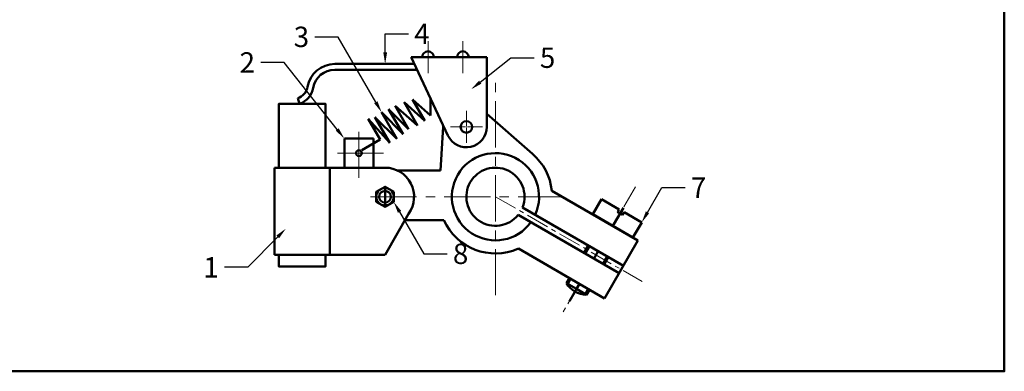
# Model space of a CAD drawing. Units: millimetres. Extents: x 77 to 718, y -35 to 313.
# Tile 4 of 7: x 379 to 718, y -35 to 86. Entities that reach past the tile are written whole.
import ezdxf
from ezdxf import colors
from ezdxf.entities.mleader import LeaderData, LeaderLine
from ezdxf.math import Vec2, Vec3

# ---------------------------------------------------------------- set-up
doc = ezdxf.new("R2010")
doc.units = ezdxf.units.MM
doc.header["$LTSCALE"] = 0.5
doc.linetypes.add('CENTER', pattern=[50.8, 31.75, -6.35, 6.35, -6.35])
for name, color, linetype, lineweight in [('M-CNTR', 1, 'CENTER', 18), ('M-OUTL', 7, 'Continuous', 50), ('M-TEXT', 3, 'Continuous', 25)]:
    doc.layers.add(name, color=color, linetype=linetype, lineweight=lineweight)
doc.styles.get("Standard").update_dxf_attribs({"font": 'arial.ttf'})

# ---------------------------------------------------------------- blocks, each defined once
blk = doc.blocks.new('*U137')
at = {"layer": 'M-CNTR', "color": 0, "transparency": 16777216}
for p, q in [((0, 0.4), (0, 5.5)), ((-5.5, 0), (-0.4, 0)), ((0.4, 0), (5.5, 0)), ((0, -5.5), (0, -0.4))]:
    blk.add_line(p, q, dxfattribs=at)
at = {"layer": 'M-CNTR', "color": 0, "linetype": 'Continuous', "transparency": 16777216}
for p, q in [((-0.2, 0), (0.2, 0)), ((0, -0.2), (0, 0.2))]:
    blk.add_line(p, q, dxfattribs=at)
blk = doc.blocks.new('*U138')
at = {"layer": 'M-CNTR', "color": 0, "transparency": 16777216}
blk.add_line((0, -8.5), (0, 8.5), dxfattribs=at)
blk = doc.blocks.new('*U139')
at = {"layer": 'M-CNTR', "color": 0, "transparency": 16777216}
blk.add_line((8.5, 0), (-8.5, 0), dxfattribs=at)
blk = doc.blocks.new('*U140')
at = {"layer": 'M-CNTR', "color": 0, "transparency": 16777216}
for p, q in [((0, 0.4), (0, 5.5)), ((-5.5, 0), (-0.4, 0)), ((0.4, 0), (5.5, 0)), ((0, -5.5), (0, -0.4))]:
    blk.add_line(p, q, dxfattribs=at)
at = {"layer": 'M-CNTR', "color": 0, "linetype": 'Continuous', "transparency": 16777216}
for p, q in [((-0.2, 0), (0.2, 0)), ((0, -0.2), (0, 0.2))]:
    blk.add_line(p, q, dxfattribs=at)
blk = doc.blocks.new('*U141')
at = {"layer": 'M-CNTR', "color": 0, "transparency": 16777216}
for p, q in [((0, 0.4), (0, 5.5)), ((-5.5, 0), (-0.4, 0)), ((0.4, 0), (5.5, 0)), ((0, -5.5), (0, -0.4))]:
    blk.add_line(p, q, dxfattribs=at)
at = {"layer": 'M-CNTR', "color": 0, "linetype": 'Continuous', "transparency": 16777216}
for p, q in [((-0.2, 0), (0.2, 0)), ((0, -0.2), (0, 0.2))]:
    blk.add_line(p, q, dxfattribs=at)
blk = doc.blocks.new('BRACKET-PLATE')
at = {"ltscale": 0.5}
for p, q in [((0, 31), (26, 31)), ((12.66, 4.03), (0, 31)), ((26, 31), (26, 7))]:
    blk.add_line(p, q, dxfattribs=at)
blk.add_arc((19, 7), 7, 205.1481, 0, dxfattribs=at)
blk = doc.blocks.new('SHUNT-TERMINAL')
for p, q in [((19.31, 22.65), (54.05, 2.6)), ((17.81, 20.06), (52.55, 0))]:
    blk.add_line(p, q)
blk.add_arc((10, 26.3), 10, 338.6269, 321.3731)

msp = doc.modelspace()

# ---------------------------------------------------------------- linework, layer by layer
at = {"layer": 'M-CNTR'}
for p, q in [((542.913, -8.747), (542.913, 64.923)), ((499.913, 25.115), (565.913, 25.115))]:
    msp.add_line(p, q, dxfattribs=at)
at = {"layer": 'M-CNTR', "ltscale": 0.5}
for p, q in [((591.064, 28.513), (583.304, 15.074)), ((542.913, 25.115), (593.347, -4.003)), ((578.304, 6.414), (576.804, 3.816)), ((571.804, -4.845), (565.828, -15.196))]:
    msp.add_line(p, q, dxfattribs=at)
at = {"layer": 'M-OUTL', "ltscale": 0.5}
for p, q in [((474.881, 58.988), (475.507, 57.089)), ((516.15, 49.564), (511.498, 57.623)), ((511.498, 57.623), (518.592, 51.218)), ((518.592, 51.218), (514.355, 58.556)), ((514.355, 58.556), (520.536, 53.037)), ((520.536, 53.037), (520.536, 59.007)), ((511.147, 46.647), (506.162, 55.281)), ((506.162, 55.281), (513.012, 48.349)), ((513.012, 48.349), (508.408, 56.324)), ((508.408, 56.324), (516.15, 49.564)), ((503.242, 44.756), (499.116, 51.902)), ((499.116, 51.902), (506.524, 43.609)), ((506.524, 43.609), (501.375, 52.528)), ((501.375, 52.528), (509.003, 45.04)), ((509.003, 45.04), (503.748, 54.142)), ((503.748, 54.142), (511.147, 46.647)), ((490.936, 45.115), (500.936, 45.115)), ((490.936, 35.115), (490.936, 45.115)), ((496.936, 41.115), (503.242, 44.756)), ((500.936, 45.115), (500.936, 35.115)), ((466.913, 35.115), (504.913, 35.115)), ((466.913, 5.115), (466.913, 35.115)), ((485.913, 5.115), (485.913, 35.115)), ((498.796, 35.115), (488.796, 35.115)), ((504.913, 28.115), (504.913, 22.115)), ((579.376, 24.27), (576.376, 19.074)), ((579.376, 24.27), (585.438, 20.77)), ((585.438, 20.77), (584.938, 19.904)), ((513.038, 19.286), (504.913, 5.115)), ((576.376, 19.074), (590.232, 11.074)), ((579.841, 17.074), (579.841, 17.074)), ((584.938, 19.904), (585.804, 19.404)), ((585.804, 19.404), (586.67, 18.904)), ((586.67, 18.904), (587.17, 19.77)), ((587.17, 19.77), (593.232, 16.27)), ((593.232, 16.27), (590.232, 11.074)), ((573.34, 5.816), (574.841, 8.414)), ((573.773, 5.566), (575.273, 8.164)), ((504.913, 5.115), (466.913, 5.115)), ((578.304, 6.414), (576.804, 3.816)), ((579.835, 2.066), (581.335, 4.664)), ((580.268, 1.816), (581.768, 4.414)), ((567.34, -4.576), (568.34, -2.844)), ((567.773, -4.826), (568.773, -3.094)), ((570.804, -6.576), (567.34, -4.576)), ((571.804, -4.844), (570.804, -6.576)), ((570.804, -6.576), (574.268, -8.576)), ((573.835, -8.326), (574.835, -6.594)), ((574.268, -8.576), (575.268, -6.844))]:
    msp.add_line(p, q, dxfattribs=at)
at = {"layer": 'M-OUTL'}
for p, q in [((539.913, 53.588), (555.721, 39.819)), ((524.913, 49.115), (523.975, 34.115)), ((509.272, 34.115), (523.975, 34.115)), ((504.913, 22.115), (504.913, 28.115)), ((562.301, 27.2), (591.964, 10.074)), ((583.304, 15.074), (586.928, 21.351)), ((511.794, 17.115), (525.13, 17.115)), ((550.801, 7.282), (580.464, -9.844)), ((580.464, -9.844), (591.964, 10.074)), ((576.804, 3.816), (578.304, 6.414)), ((568.393, -10.752), (571.804, -4.844))]:
    msp.add_line(p, q, dxfattribs=at)
at = {"layer": 'M-OUTL', "ltscale": 0.5}
for points in [[(77.418, 312.912), (718.012, 312.912), (718.012, -34.898), (77.418, -34.898)], [(507.913, 26.847), (504.913, 28.579), (501.913, 26.847), (501.913, 23.383), (504.913, 21.651), (507.913, 23.383)]]:
    msp.add_lwpolyline(points, close=True, dxfattribs=at)
for points in [[(474.881, 58.988, 0.2770282), (478.242, 62.884, -0.3648802), (487.603, 70.765), (515.016, 70.765)], [(475.507, 57.089, 0.2770282), (480.213, 62.543, -0.3648802), (487.603, 68.765), (515.955, 68.765)]]:
    msp.add_lwpolyline(points, format="xyb", dxfattribs=at)
for points in [[(468.415, 35.146), (468.415, 57.089), (484.415, 57.089), (484.415, 35.146)], [(484.413, 5.115), (484.413, 1.115), (468.413, 1.115), (468.413, 5.115)]]:
    msp.add_lwpolyline(points, dxfattribs=at)
at = {"layer": 'M-OUTL'}
for centre, radius in [((532.913, 49.115), 2), ((504.913, 25.115), 3)]:
    msp.add_circle(centre, radius, dxfattribs=at)
at = {"layer": 'M-OUTL', "ltscale": 0.5}
for centre, radius in [((495.936, 40.115), 1), ((504.913, 25.115), 3), ((504.913, 25.115), 2)]:
    msp.add_circle(centre, radius, dxfattribs=at)
for centre, radius, start, end in [((519.707, 73.115), 2, 0, 180), ((531.707, 73.115), 2, 0, 180), ((504.913, 25.115), 10, 324.34264, 90), ((574.268, -0.576), 8, 209.99853, 269.99853)]:
    msp.add_arc(centre, radius, start, end, dxfattribs=at)
at = {"layer": 'M-OUTL'}
for centre, radius, start, end in [((532.913, 49.115), 8, 176.19309, 180), ((542.913, 25.115), 15, 335.73917, 324.26083), ((542.913, 25.115), 19.5, 6.13881, 48.94259), ((542.913, 25.115), 19.5, 204.22094, 293.86119)]:
    msp.add_arc(centre, radius, start, end, dxfattribs=at)

# ---------------------------------------------------------------- block references
at = {"layer": 'M-CNTR'}
for name, p in [('*U141', (519.707, 73.115)), ('*U140', (531.707, 73.115)), ('*U137', (532.913, 49.115)), ('*U138', (495.936, 40.115)), ('*U139', (495.936, 40.115))]:
    msp.add_blockref(name, p, dxfattribs=at)
at = {"layer": 'M-OUTL'}
for name, p in [('BRACKET-PLATE', (513.913, 42.114)), ('SHUNT-TERMINAL', (532.912, -1.184))]:
    msp.add_blockref(name, p, dxfattribs=at)

# ---------------------------------------------------------------- leaders
at = {"layer": 'M-TEXT', "ltscale": 0.5}
ml = msp.add_multileader_mtext('Standard', dxfattribs=at)
ml.set_content('3', color=256)
ml.set_leader_properties()
ml.build(insert=Vec2(0, 0))
ctx = ml.context
ctx.base_point, ctx.char_height, ctx.plane_origin = Vec3(472.218, 80.028), 7, Vec3(503.748, 54.142)
ctx.text_align_type = 2
notes = []
notes.append((ctx, [(0, (1, 1, 0), (488.802, 80.028), (-1, 0), 8, [(0, [(503.748, 54.142)], 0, [])])]))
ctx.mtext.insert, ctx.mtext.alignment, ctx.mtext.flow_direction = Vec3(478.802, 83.59), 3, 5
ml = msp.add_multileader_mtext('Standard', dxfattribs=at)
ml.set_content('4', color=256)
ml.set_leader_properties()
ml.build(insert=Vec2(0, 0))
ctx = ml.context
ctx.base_point, ctx.char_height, ctx.plane_origin = Vec3(512.971, 81.15), 7, Vec3(504.971, 70.765)
notes.append((ctx, [(0, (1, 1, 0), (504.971, 81.15), (1, 0), 8, [(0, [(504.971, 70.765)], 0, [])])]))
ctx.mtext.insert, ctx.mtext.flow_direction = Vec3(514.971, 84.65), 5
ml = msp.add_multileader_mtext('Standard', dxfattribs=at)
ml.set_content('2', color=256)
ml.set_leader_properties()
ml.build(insert=Vec2(0, 0))
ctx = ml.context
ctx.base_point, ctx.char_height, ctx.plane_origin = Vec3(453.544, 71.297), 7, Vec3(490.936, 45.115)
ctx.text_align_type = 2
notes.append((ctx, [(0, (1, 1, 0), (470.18, 71.297), (-1, 0), 8, [(0, [(490.936, 45.115)], 0, [])])]))
ctx.mtext.insert, ctx.mtext.alignment, ctx.mtext.flow_direction = Vec3(460.18, 74.797), 3, 5
ml = msp.add_multileader_mtext('Standard', dxfattribs=at)
ml.set_content('5', color=256)
ml.set_leader_properties()
ml.build(insert=Vec2(0, 0))
ctx = ml.context
ctx.base_point, ctx.char_height, ctx.plane_origin = Vec3(556.208, 72.856), 7, Vec3(534.535, 62.038)
notes.append((ctx, [(0, (1, 1, 0), (548.208, 72.856), (1, 0), 8, [(0, [(534.535, 62.038)], 0, [])])]))
ctx.mtext.insert, ctx.mtext.flow_direction = Vec3(558.208, 76.416), 5
ml = msp.add_multileader_mtext('Standard', dxfattribs=at)
ml.set_content('7', color=256)
ml.set_leader_properties()
ml.build(insert=Vec2(0, 0))
ctx = ml.context
ctx.base_point, ctx.char_height, ctx.plane_origin = Vec3(608.142, 28.239), 7, Vec3(593.232, 16.27)
notes.append((ctx, [(0, (1, 1, 0), (600.142, 28.239), (1, 0), 8, [(0, [(593.232, 16.27)], 0, [])])]))
ctx.mtext.insert, ctx.mtext.flow_direction = Vec3(610.142, 31.739), 5
ml = msp.add_multileader_mtext('Standard', dxfattribs=at)
ml.set_content('8', color=256)
ml.set_leader_properties()
ml.build(insert=Vec2(0, 0))
ctx = ml.context
ctx.base_point, ctx.char_height, ctx.plane_origin = Vec3(526.277, 5.432), 7, Vec3(507.913, 23.383)
notes.append((ctx, [(0, (1, 1, 0), (518.277, 5.432), (1, 0), 8, [(0, [(507.913, 23.383)], 0, [])])]))
ctx.mtext.insert, ctx.mtext.flow_direction = Vec3(528.277, 8.991), 5
ml = msp.add_multileader_mtext('Standard', dxfattribs=at)
ml.set_content('1', color=256)
ml.set_leader_properties()
ml.build(insert=Vec2(0, 0))
ctx = ml.context
ctx.base_point, ctx.char_height, ctx.plane_origin = Vec3(443.115, 0.849), 7, Vec3(470.819, 14.181)
ctx.text_align_type = 2
notes.append((ctx, [(0, (1, 1, 0), (457.694, 0.849), (-1, 0), 8, [(0, [(470.819, 14.181)], 0, [])])]))
ctx.mtext.insert, ctx.mtext.alignment, ctx.mtext.flow_direction = Vec3(447.694, 4.349), 3, 5
for ctx, leaders in notes:
    for number, flags, end, landing, length, lines in leaders:
        leader = LeaderData()
        leader.index, (leader.has_last_leader_line, leader.has_dogleg_vector, leader.attachment_direction) = number, flags
        leader.last_leader_point, leader.dogleg_vector, leader.dogleg_length = Vec3(end), Vec3(landing), length
        for number, points, colour, breaks in lines:
            line = LeaderLine()
            line.index, line.vertices, line.color, line.breaks = number, Vec3.list(points), colors.encode_raw_color(colour), breaks
            leader.lines.append(line)
        ctx.leaders.append(leader)

doc.saveas('drawing.dxf')
